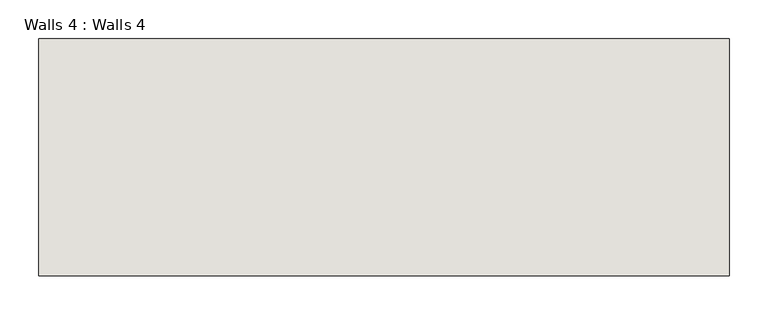
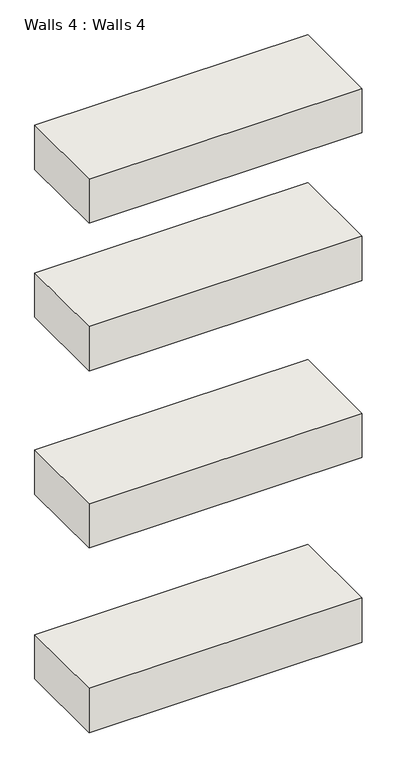
"""IFC4 building model written with IfcOpenShell, lengths in millimetres: wall geometry, Walls 4 : Walls 4."""

from ifc_helpers import new_model, si_unit, frame, origin, place, context, project, spatial, polyline, outline, extrude, source, transform, mapped, element, save


def walls_4_walls_4_61d7950c(model_context):
    return source(origin(), model_context, "Body", "SweptSolid", [
        extrude(outline(polyline([(-6445.0514478, 3656.1956099), (-7334.0514478, 3656.1956099), (-7334.0514478, 3960.9956099), (-6445.0514478, 3960.9956099), (-6445.0514478, 3656.1956099)])), frame((0.0, 0.0, 304.0861818), z_axis=(0.0, 0.0, 1.0), x_axis=(1.0, 0.0, 0.0)), (0.0, 0.0, 1.0), 152.4),
        extrude(outline(polyline([(-6445.0514478, 3656.1956099), (-7334.0514478, 3656.1956099), (-7334.0514478, 3960.9956099), (-6445.0514478, 3960.9956099), (-6445.0514478, 3656.1956099)])), frame((0.0, 0.0, 939.0861818), z_axis=(0.0, 0.0, 1.0), x_axis=(1.0, 0.0, 0.0)), (0.0, 0.0, 1.0), 152.4),
        extrude(outline(polyline([(-6445.0514478, 3656.1956099), (-7334.0514478, 3656.1956099), (-7334.0514478, 3960.9956099), (-6445.0514478, 3960.9956099), (-6445.0514478, 3656.1956099)])), frame((0.0, 0.0, 1548.6861818), z_axis=(0.0, 0.0, 1.0), x_axis=(1.0, 0.0, 0.0)), (0.0, 0.0, 1.0), 152.4),
        extrude(outline(polyline([(-6445.0514478, 3656.1956099), (-7334.0514478, 3656.1956099), (-7334.0514478, 3960.9956099), (-6445.0514478, 3960.9956099), (-6445.0514478, 3656.1956099)])), frame((0.0, 0.0, 2056.6861818), z_axis=(0.0, 0.0, 1.0), x_axis=(1.0, 0.0, 0.0)), (0.0, 0.0, 1.0), 152.4),
    ])


if __name__ == "__main__":
    model = new_model("IFC4")
    model_context = context("Model", 3, world=origin())
    ifc_project = project(units=[si_unit("LENGTHUNIT", "METRE", prefix="MILLI")], contexts=[model_context])
    site = spatial("IfcSite", under=ifc_project)
    building = spatial("IfcBuilding", under=site)
    placement = place(None, origin())
    walls_4_walls_4_shape = walls_4_walls_4_61d7950c(model_context)
    element("IfcWall", 1, ObjectType="Walls 4 : Walls 4", at=placement, inside=building, context=model_context, shape_type="MappedRepresentation", body=[
        mapped(walls_4_walls_4_shape, transform((0.0, 0.0, 0.0), x_axis=(1.0, 0.0, 0.0), y_axis=(0.0, 1.0, 0.0), z_axis=(0.0, 0.0, 1.0))),
    ])
    save(model, "model.ifc")

# Revit data of these elements
# Element 1 (IfcWall, "Walls 4 : Walls 4")
#   Materials on its faces: "Default Wall"
# Materials
#   "Default Wall": colour RGB 80 80 80, transparency 0
